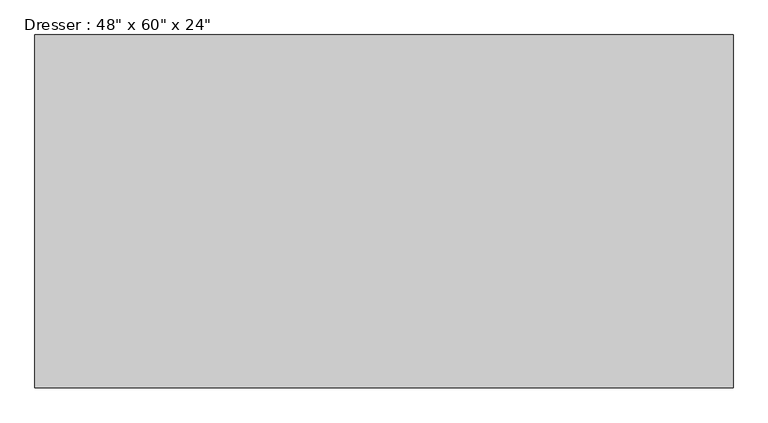
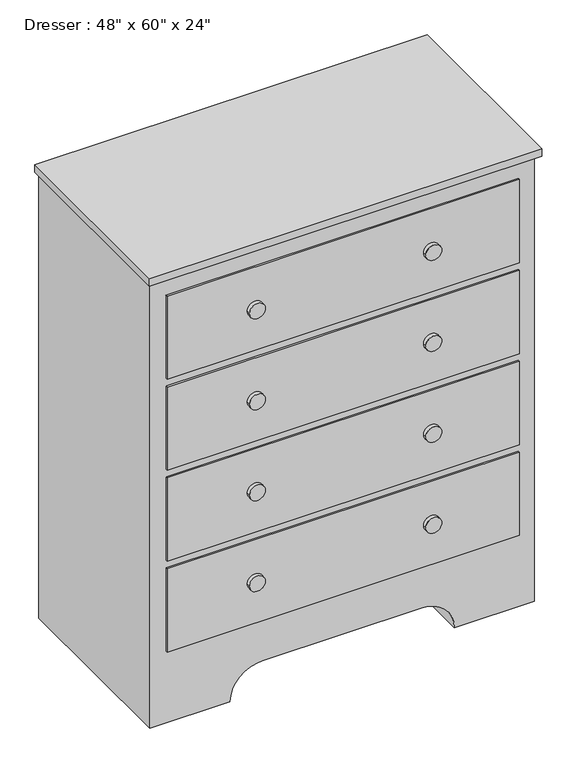
"""IFC4 building model written with IfcOpenShell, lengths in millimetres: furniture geometry."""

from ifc_helpers import new_model, si_unit, point, frame, frame_2d, origin, place, context, project, spatial, polyline, circle_curve, trimmed, segment, composite_curve, outline, extrude, source, transform, mapped, element, save


def furniture_2babcf72(model_context):
    return source(origin(), model_context, "Body", "SweptSolid", [
        extrude(outline(polyline([(353.1067402, -58.3629541), (353.1067402, -687.0129541), (-891.4932598, -687.0129541), (-891.4932598, -58.3629541), (353.1067402, -58.3629541)])), frame((0.0, 0.0, 1498.6), z_axis=(0.0, 0.0, 1.0), x_axis=(1.0, 0.0, 0.0)), (0.0, 0.0, 1.0), 25.4),
        extrude(outline(composite_curve([segment(polyline([(0.0, 340.4067402), (1498.6, 340.4067402), (1498.6, -878.7932598), (0.0, -878.7932598), (0.0, -624.7932598)]), True, "CONTINUOUS"), segment(trimmed(circle_curve(frame_2d((0.0, -523.1932598)), 101.6), [point((0.0, -624.7932598))], [point((101.6, -523.1932598))], True, "CARTESIAN"), True, "CONTINUOUS"), segment(polyline([(101.6, -523.1932598), (101.6, -15.1932598)]), True, "CONTINUOUS"), segment(trimmed(circle_curve(frame_2d((0.0, -15.1932598)), 101.6), [point((101.6, -15.1932598))], [point((0.0, 86.4067402))], True, "CARTESIAN"), True, "CONTINUOUS"), segment(polyline([(0.0, 86.4067402), (0.0, 340.4067402)]), True, "CONTINUOUS")], self_intersect=False)), frame((0.0, -667.9629541, 0.0), z_axis=(0.0, 1.0, 0.0), x_axis=(0.0, 0.0, 1.0)), (0.0, 0.0, 1.0), 609.6),
        extrude(outline(composite_curve([segment(trimmed(circle_curve(frame_2d((1295.4, 10.2067402)), 25.4), [point((1295.4, -15.1932598))], [point((1295.4, 35.6067402))], False, "CARTESIAN"), True, "CONTINUOUS"), segment(trimmed(circle_curve(frame_2d((1295.4, 10.2067402)), 25.4), [point((1295.4, 35.6067402))], [point((1295.4, -15.1932598))], False, "CARTESIAN"), True, "CONTINUOUS")], self_intersect=False)), frame((0.0, -687.0129541, 0.0), z_axis=(0.0, 1.0, 0.0), x_axis=(0.0, 0.0, 1.0)), (0.0, 0.0, 1.0), 12.7),
        extrude(outline(composite_curve([segment(trimmed(circle_curve(frame_2d((990.6, 10.2067402)), 25.4), [point((990.6, -15.1932598))], [point((990.6, 35.6067402))], False, "CARTESIAN"), True, "CONTINUOUS"), segment(trimmed(circle_curve(frame_2d((990.6, 10.2067402)), 25.4), [point((990.6, 35.6067402))], [point((990.6, -15.1932598))], False, "CARTESIAN"), True, "CONTINUOUS")], self_intersect=False)), frame((0.0, -687.0129541, 0.0), z_axis=(0.0, 1.0, 0.0), x_axis=(0.0, 0.0, 1.0)), (0.0, 0.0, 1.0), 12.7),
        extrude(outline(composite_curve([segment(trimmed(circle_curve(frame_2d((685.8, 10.2067402)), 25.4), [point((685.8, -15.1932598))], [point((685.8, 35.6067402))], False, "CARTESIAN"), True, "CONTINUOUS"), segment(trimmed(circle_curve(frame_2d((685.8, 10.2067402)), 25.4), [point((685.8, 35.6067402))], [point((685.8, -15.1932598))], False, "CARTESIAN"), True, "CONTINUOUS")], self_intersect=False)), frame((0.0, -687.0129541, 0.0), z_axis=(0.0, 1.0, 0.0), x_axis=(0.0, 0.0, 1.0)), (0.0, 0.0, 1.0), 12.7),
        extrude(outline(composite_curve([segment(trimmed(circle_curve(frame_2d((381.0, 10.2067402)), 25.4), [point((381.0, -15.1932598))], [point((381.0, 35.6067402))], False, "CARTESIAN"), True, "CONTINUOUS"), segment(trimmed(circle_curve(frame_2d((381.0, 10.2067402)), 25.4), [point((381.0, 35.6067402))], [point((381.0, -15.1932598))], False, "CARTESIAN"), True, "CONTINUOUS")], self_intersect=False)), frame((0.0, -687.0129541, 0.0), z_axis=(0.0, 1.0, 0.0), x_axis=(0.0, 0.0, 1.0)), (0.0, 0.0, 1.0), 12.7),
        extrude(outline(composite_curve([segment(trimmed(circle_curve(frame_2d((381.0, -548.5932598)), 25.4), [point((381.0, -573.9932598))], [point((381.0, -523.1932598))], False, "CARTESIAN"), True, "CONTINUOUS"), segment(trimmed(circle_curve(frame_2d((381.0, -548.5932598)), 25.4), [point((381.0, -523.1932598))], [point((381.0, -573.9932598))], False, "CARTESIAN"), True, "CONTINUOUS")], self_intersect=False)), frame((0.0, -687.0129541, 0.0), z_axis=(0.0, 1.0, 0.0), x_axis=(0.0, 0.0, 1.0)), (0.0, 0.0, 1.0), 12.7),
        extrude(outline(composite_curve([segment(trimmed(circle_curve(frame_2d((685.8, -548.5932598)), 25.4), [point((685.8, -573.9932598))], [point((685.8, -523.1932598))], False, "CARTESIAN"), True, "CONTINUOUS"), segment(trimmed(circle_curve(frame_2d((685.8, -548.5932598)), 25.4), [point((685.8, -523.1932598))], [point((685.8, -573.9932598))], False, "CARTESIAN"), True, "CONTINUOUS")], self_intersect=False)), frame((0.0, -687.0129541, 0.0), z_axis=(0.0, 1.0, 0.0), x_axis=(0.0, 0.0, 1.0)), (0.0, 0.0, 1.0), 12.7),
        extrude(outline(composite_curve([segment(trimmed(circle_curve(frame_2d((990.6, -548.5932598)), 25.4), [point((990.6, -573.9932598))], [point((990.6, -523.1932598))], False, "CARTESIAN"), True, "CONTINUOUS"), segment(trimmed(circle_curve(frame_2d((990.6, -548.5932598)), 25.4), [point((990.6, -523.1932598))], [point((990.6, -573.9932598))], False, "CARTESIAN"), True, "CONTINUOUS")], self_intersect=False)), frame((0.0, -687.0129541, 0.0), z_axis=(0.0, 1.0, 0.0), x_axis=(0.0, 0.0, 1.0)), (0.0, 0.0, 1.0), 12.7),
        extrude(outline(composite_curve([segment(trimmed(circle_curve(frame_2d((1295.4, -548.5932598)), 25.4), [point((1295.4, -573.9932598))], [point((1295.4, -523.1932598))], False, "CARTESIAN"), True, "CONTINUOUS"), segment(trimmed(circle_curve(frame_2d((1295.4, -548.5932598)), 25.4), [point((1295.4, -523.1932598))], [point((1295.4, -573.9932598))], False, "CARTESIAN"), True, "CONTINUOUS")], self_intersect=False)), frame((0.0, -687.0129541, 0.0), z_axis=(0.0, 1.0, 0.0), x_axis=(0.0, 0.0, 1.0)), (0.0, 0.0, 1.0), 12.7),
        extrude(outline(polyline([(289.6067402, -674.3129541), (-827.9932598, -674.3129541), (-827.9932598, -667.9629541), (289.6067402, -667.9629541), (289.6067402, -674.3129541)])), frame((0.0, 0.0, 1155.7), z_axis=(0.0, 0.0, 1.0), x_axis=(1.0, 0.0, 0.0)), (0.0, 0.0, 1.0), 279.4),
        extrude(outline(polyline([(289.6067402, -674.3129541), (-827.9932598, -674.3129541), (-827.9932598, -667.9629541), (289.6067402, -667.9629541), (289.6067402, -674.3129541)])), frame((0.0, 0.0, 850.9), z_axis=(0.0, 0.0, 1.0), x_axis=(1.0, 0.0, 0.0)), (0.0, 0.0, 1.0), 279.4),
        extrude(outline(polyline([(289.6067402, -674.3129541), (-827.9932598, -674.3129541), (-827.9932598, -667.9629541), (289.6067402, -667.9629541), (289.6067402, -674.3129541)])), frame((0.0, 0.0, 546.1), z_axis=(0.0, 0.0, 1.0), x_axis=(1.0, 0.0, 0.0)), (0.0, 0.0, 1.0), 279.4),
        extrude(outline(polyline([(289.6067402, -674.3129541), (-827.9932598, -674.3129541), (-827.9932598, -667.9629541), (289.6067402, -667.9629541), (289.6067402, -674.3129541)])), frame((0.0, 0.0, 241.3), z_axis=(0.0, 0.0, 1.0), x_axis=(1.0, 0.0, 0.0)), (0.0, 0.0, 1.0), 279.4),
    ])


if __name__ == "__main__":
    model = new_model("IFC4")
    model_context = context("Model", 3, world=origin())
    ifc_project = project(units=[si_unit("LENGTHUNIT", "METRE", prefix="MILLI")], contexts=[model_context])
    site = spatial("IfcSite", under=ifc_project)
    building = spatial("IfcBuilding", under=site)
    placement = place(None, origin())
    furniture_shape = furniture_2babcf72(model_context)
    element("IfcFurniture", 1, ObjectType="Dresser : 48\" x 60\" x 24\"", at=placement, inside=building, context=model_context, shape_type="MappedRepresentation", body=[
        mapped(furniture_shape, transform((0.0, 0.0, 0.0), x_axis=(1.0, 0.0, 0.0), y_axis=(0.0, 1.0, 0.0), z_axis=(0.0, 0.0, 1.0))),
    ])
    save(model, "model.ifc")

# Revit data of these elements
# Type "Dresser : 48\" x 60\" x 24\""
#   Assembly Code = "E2020200"
#   Depth = 2' - 0"
#   Height = 5' - 0"
#   Width = 4' - 0"
#   Dresser Material = Laminate - Ivory, Glossy
#   Drawer Material = Laminate, Ivory, Matte
#   Knob Material = Cherry
#   Default Elevation = 0
# Element 1 (IfcFurniture, "Dresser : 48\" x 60\" x 24\"")
#   Materials on its faces: "Laminate, Ivory, Matte", "Cherry", "Laminate - Ivory, Glossy"
# Materials
#   "Laminate - Ivory, Glossy": colour RGB 247 247 239, transparency 0
#   "Laminate, Ivory, Matte": class "Plastic", colour RGB 247 247 239, transparency 0, Description = "Plastic Laminate - Ivory, Matte", Cost = 0
#   "Cherry": class "Wood", colour RGB 226 177 128, transparency 0, Description = "Prunus Serotina", Cost = 0
